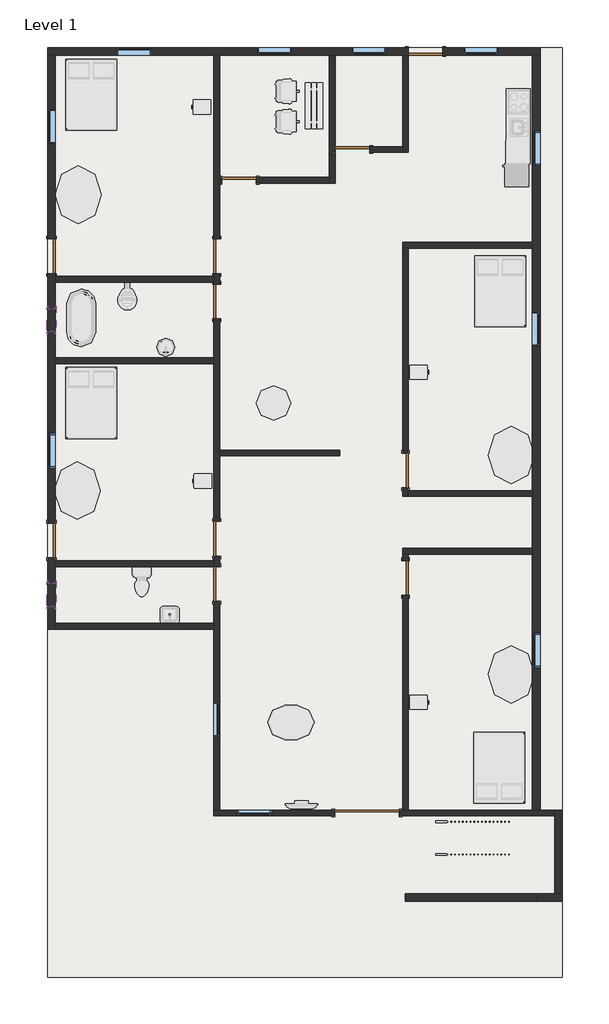
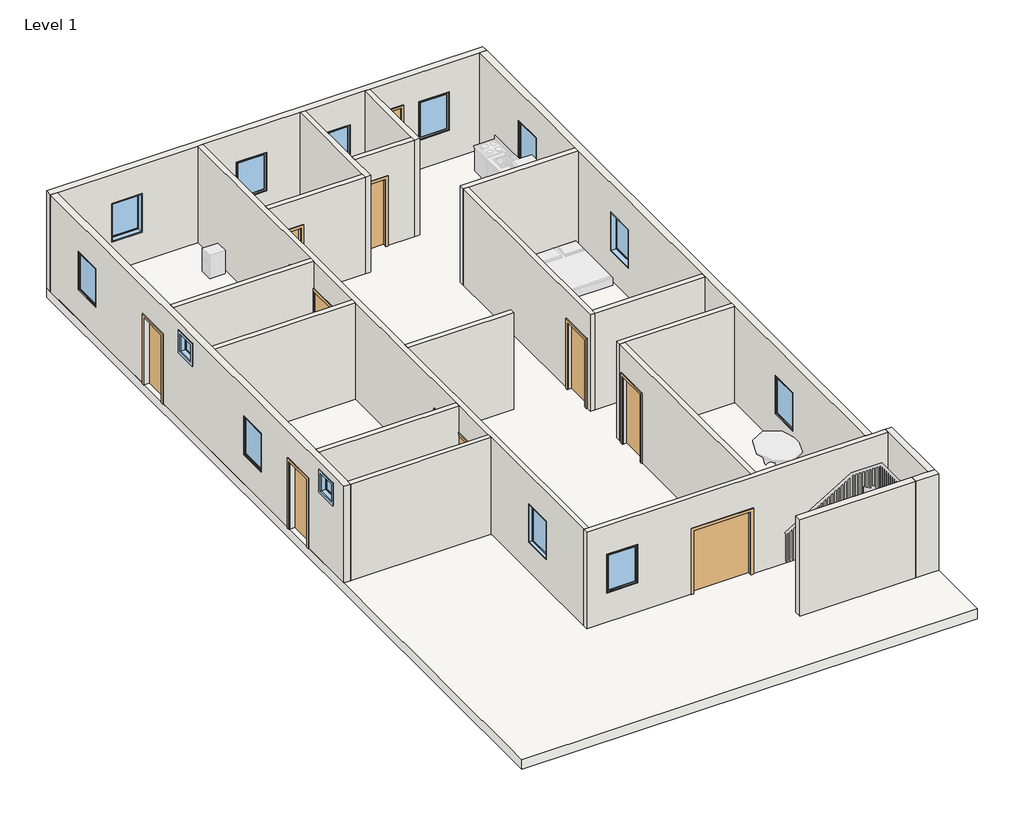
# One storey, part 1 of 2: 22 walls, 13 windows, 12 doors, 1 slab.
"""IFC4 building model written with IfcOpenShell, lengths in millimetres."""

from ifc_helpers import new_model, si_unit, frame, origin, origin_with_axes, place, context, project, spatial, polyline, outline, extrude, faceted_brep, transform, mapped, element, save
from components import m_door_double_flush_panel_double_acting_1700_x_2000mm_82a3dfda, door_54dd4da4, door_686f89d2, door_16372e1c, window_e2841890, window_d657a5cb, window_e41d21a6

model = new_model("IFC4")

# Units and contexts
model_context = context("Model", 3, world=origin())
ifc_project = project(units=[si_unit("LENGTHUNIT", "METRE", prefix="MILLI")], contexts=[model_context])

# Site, building, storey
site = spatial("IfcSite", under=ifc_project)
building = spatial("IfcBuilding", under=site)
storey = spatial("IfcBuildingStorey", under=building, Name="Level 1", Elevation=0.0)

# Doors
placement = place(None, origin())
m_door_double_flush_panel_double_acting_1700_x_2000mm_shape = m_door_double_flush_panel_double_acting_1700_x_2000mm_82a3dfda(model_context)
element("IfcDoor", 1, ObjectType="M_Door-Double-Flush_Panel-Double-Acting : 1700 x 2000mm", at=placement, inside=storey, context=model_context, shape_type="MappedRepresentation", body=[
    mapped(m_door_double_flush_panel_double_acting_1700_x_2000mm_shape, transform((-10492.7409023, -9232.8133562, 0.0), x_axis=(1.0, 0.0, 0.0), y_axis=(0.0, 1.0, 0.0), z_axis=(0.0, 0.0, 1.0))),
])
door_shape = door_54dd4da4(model_context)
element("IfcDoor", 2, ObjectType="Single-Flush : 36\" x 84\"", at=placement, inside=storey, context=model_context, shape_type="MappedRepresentation", body=[
    mapped(door_shape, transform((-18823.9409023, 5462.5226537, 0.0), x_axis=(0.0, -1.0, 0.0), y_axis=(1.0, 0.0, 0.0), z_axis=(0.0, 0.0, 1.0))),
])
element("IfcDoor", 3, ObjectType="Single-Flush : 36\" x 84\"", at=placement, inside=storey, context=model_context, shape_type="MappedRepresentation", body=[
    mapped(door_shape, transform((-8943.3409023, 10872.7226537, 0.0), x_axis=(-1.0, 0.0, 0.0), y_axis=(0.0, -1.0, 0.0), z_axis=(0.0, 0.0, 1.0))),
])
element("IfcDoor", 4, ObjectType="Single-Flush : 36\" x 84\"", at=placement, inside=storey, context=model_context, shape_type="MappedRepresentation", body=[
    mapped(door_shape, transform((-18823.9409023, -2044.6133562, 0.0), x_axis=(0.0, -1.0, 0.0), y_axis=(1.0, 0.0, 0.0), z_axis=(0.0, 0.0, 1.0))),
])
door_2_shape = door_686f89d2(model_context)
element("IfcDoor", 5, ObjectType="Single-Flush : 36\" x 84\"", at=placement, inside=storey, context=model_context, shape_type="MappedRepresentation", body=[
    mapped(door_2_shape, transform((-14455.1409023, 5462.5226537, 0.0), x_axis=(0.0, -1.0, 0.0), y_axis=(1.0, 0.0, 0.0), z_axis=(0.0, 0.0, 1.0))),
])
element("IfcDoor", 6, ObjectType="Single-Flush : 36\" x 84\"", at=placement, inside=storey, context=model_context, shape_type="MappedRepresentation", body=[
    mapped(door_2_shape, transform((-13870.9409023, 7469.1226537, 0.0), x_axis=(-1.0, 0.0, 0.0), y_axis=(0.0, -1.0, 0.0), z_axis=(0.0, 0.0, 1.0))),
])
element("IfcDoor", 7, ObjectType="Single-Flush : 36\" x 84\"", at=placement, inside=storey, context=model_context, shape_type="MappedRepresentation", body=[
    mapped(door_2_shape, transform((-10873.7409023, 8281.9226537, 0.0), x_axis=(-1.0, 0.0, 0.0), y_axis=(0.0, -1.0, 0.0), z_axis=(0.0, 0.0, 1.0))),
])
element("IfcDoor", 8, ObjectType="Single-Flush : 36\" x 84\"", at=placement, inside=storey, context=model_context, shape_type="MappedRepresentation", body=[
    mapped(door_2_shape, transform((-14455.1409023, -1993.8133562, 0.0), x_axis=(0.0, -1.0, 0.0), y_axis=(1.0, 0.0, 0.0), z_axis=(0.0, 0.0, 1.0))),
])
element("IfcDoor", 9, ObjectType="Single-Flush : 36\" x 84\"", at=placement, inside=storey, context=model_context, shape_type="MappedRepresentation", body=[
    mapped(door_2_shape, transform((-9476.7409023, -3035.2133562, 0.0), x_axis=(0.0, 1.0, 0.0), y_axis=(-1.0, 0.0, 0.0), z_axis=(0.0, 0.0, 1.0))),
])
door_3_shape = door_16372e1c(model_context)
element("IfcDoor", 10, ObjectType="Single-Flush : 36\" x 84\"", at=placement, inside=storey, context=model_context, shape_type="MappedRepresentation", body=[
    mapped(door_3_shape, transform((-9476.7409023, -190.4133562, 0.0), x_axis=(0.0, -1.0, 0.0), y_axis=(1.0, 0.0, 0.0), z_axis=(0.0, 0.0, 1.0))),
])
element("IfcDoor", 11, ObjectType="Single-Flush : 36\" x 84\"", at=placement, inside=storey, context=model_context, shape_type="MappedRepresentation", body=[
    mapped(door_3_shape, transform((-14455.1409023, 4268.7226537, 0.0), x_axis=(0.0, 1.0, 0.0), y_axis=(-1.0, 0.0, 0.0), z_axis=(0.0, 0.0, 1.0))),
])
element("IfcDoor", 12, ObjectType="Single-Flush : 36\" x 84\"", at=placement, inside=storey, context=model_context, shape_type="MappedRepresentation", body=[
    mapped(door_3_shape, transform((-14455.1409023, -3187.6133562, 0.0), x_axis=(0.0, 1.0, 0.0), y_axis=(-1.0, 0.0, 0.0), z_axis=(0.0, 0.0, 1.0))),
])

# Slab
element("IfcSlab", 13, ObjectType="Generic - 12\"", at=placement, inside=storey, context=model_context, shape_type="SweptSolid", body=[
    extrude(outline(polyline([(-5336.5409023, 10974.3226537), (-5336.5409023, -13576.2133562), (-18925.5409023, -13576.2133562), (-18925.5409023, 10974.3226537), (-5336.5409023, 10974.3226537)])), frame((0.0, 0.0, -304.8), z_axis=(0.0, 0.0, 1.0), x_axis=(1.0, 0.0, 0.0)), (0.0, 0.0, 1.0), 304.8),
])

# Walls
element("IfcWall", 14, ObjectType="Generic - 8\"", at=placement, inside=storey, context=model_context, shape_type="Brep", body=[
    faceted_brep([(-18925.5409023, 10771.1226537, 0.0), (-18722.3409023, 10771.1226537, 0.0), (-14531.3409023, 10771.1226537, 0.0), (-14378.9409023, 10771.1226537, 0.0), (-11483.3409023, 10771.1226537, 0.0), (-11330.9409023, 10771.1226537, 0.0), (-9552.9409023, 10771.1226537, 0.0), (-9400.5409023, 10771.1226537, 0.0), (-9400.5409023, 10771.1226537, 2133.6), (-8486.1409023, 10771.1226537, 2133.6), (-8486.1409023, 10771.1226537, 0.0), (-6123.9409023, 10771.1226537, 0.0), (-5920.7409023, 10771.1226537, 0.0), (-5920.7409023, 10771.1226537, 3048.0), (-6123.9409023, 10771.1226537, 3048.0), (-9400.5409023, 10771.1226537, 3048.0), (-9552.9409023, 10771.1226537, 3048.0), (-11330.9409023, 10771.1226537, 3048.0), (-11483.3409023, 10771.1226537, 3048.0), (-14378.9409023, 10771.1226537, 3048.0), (-14531.3409023, 10771.1226537, 3048.0), (-18722.3409023, 10771.1226537, 3048.0), (-18925.5409023, 10771.1226537, 3048.0), (-16182.3409023, 10771.1226537, 2133.6), (-16182.3409023, 10771.1226537, 914.4), (-17096.7409023, 10771.1226537, 914.4), (-17096.7409023, 10771.1226537, 2133.6), (-13388.3409023, 10771.1226537, 2133.6), (-12473.9409023, 10771.1226537, 2133.6), (-12473.9409023, 10771.1226537, 914.4), (-13388.3409023, 10771.1226537, 914.4), (-10899.1409023, 10771.1226537, 2133.6), (-9984.7409023, 10771.1226537, 2133.6), (-9984.7409023, 10771.1226537, 914.4), (-10899.1409023, 10771.1226537, 914.4), (-7940.0409023, 10771.1226537, 2133.6), (-7025.6409023, 10771.1226537, 2133.6), (-7025.6409023, 10771.1226537, 914.4), (-7940.0409023, 10771.1226537, 914.4), (-9400.5409023, 10974.3226537, 2133.6), (-9400.5409023, 10974.3226537, 0.0), (-18925.5409023, 10974.3226537, 0.0), (-18925.5409023, 10974.3226537, 3048.0), (-5920.7409023, 10974.3226537, 3048.0), (-5920.7409023, 10974.3226537, 0.0), (-8486.1409023, 10974.3226537, 0.0), (-8486.1409023, 10974.3226537, 2133.6), (-16182.3409023, 10974.3226537, 2133.6), (-17096.7409023, 10974.3226537, 2133.6), (-17096.7409023, 10974.3226537, 914.4), (-16182.3409023, 10974.3226537, 914.4), (-13388.3409023, 10974.3226537, 2133.6), (-13388.3409023, 10974.3226537, 914.4), (-12473.9409023, 10974.3226537, 914.4), (-12473.9409023, 10974.3226537, 2133.6), (-10899.1409023, 10974.3226537, 2133.6), (-10899.1409023, 10974.3226537, 914.4), (-9984.7409023, 10974.3226537, 914.4), (-9984.7409023, 10974.3226537, 2133.6), (-7940.0409023, 10974.3226537, 2133.6), (-7940.0409023, 10974.3226537, 914.4), (-7025.6409023, 10974.3226537, 914.4), (-7025.6409023, 10974.3226537, 2133.6)], [[[0, 1, 2, 3, 4, 5, 6, 7, 8, 9, 10, 11, 12, 13, 14, 15, 16, 17, 18, 19, 20, 21, 22], [23, 24, 25, 26], [27, 28, 29, 30], [31, 32, 33, 34], [35, 36, 37, 38]], [[39, 40, 41, 42, 43, 44, 45, 46], [47, 48, 49, 50], [51, 52, 53, 54], [55, 56, 57, 58], [59, 60, 61, 62]], [[45, 44, 12, 11, 10]], [[41, 40, 7, 6, 5, 4, 3, 2, 1, 0]], [[22, 21, 20, 19, 18, 17, 16, 15, 14, 13, 43, 42]], [[0, 22, 42, 41]], [[13, 12, 44, 43]], [[8, 7, 40, 39]], [[9, 8, 39, 46]], [[10, 9, 46, 45]], [[24, 23, 47, 50]], [[25, 24, 50, 49]], [[26, 25, 49, 48]], [[23, 26, 48, 47]], [[52, 51, 27, 30]], [[53, 52, 30, 29]], [[54, 53, 29, 28]], [[51, 54, 28, 27]], [[56, 55, 31, 34]], [[57, 56, 34, 33]], [[58, 57, 33, 32]], [[55, 58, 32, 31]], [[60, 59, 35, 38]], [[61, 60, 38, 37]], [[62, 61, 37, 36]], [[59, 62, 36, 35]]]),
])
element("IfcWall", 15, ObjectType="Generic - 8\"", at=placement, inside=storey, context=model_context, shape_type="Brep", body=[
    faceted_brep([(-18925.5409023, -2501.8133562, 2133.6), (-18925.5409023, -2501.8133562, 0.0), (-18925.5409023, -4381.4133562, 0.0), (-18925.5409023, -4381.4133562, 3048.0), (-18925.5409023, 10771.1226537, 3048.0), (-18925.5409023, 10771.1226537, 0.0), (-18925.5409023, 5919.7226537, 0.0), (-18925.5409023, 5919.7226537, 2133.6), (-18925.5409023, 5005.3226537, 2133.6), (-18925.5409023, 5005.3226537, 0.0), (-18925.5409023, -1587.4133562, 0.0), (-18925.5409023, -1587.4133562, 2133.6), (-18925.5409023, 9348.7226537, 2133.6), (-18925.5409023, 8434.3226537, 2133.6), (-18925.5409023, 8434.3226537, 914.4), (-18925.5409023, 9348.7226537, 914.4), (-18925.5409023, 787.4866438, 2133.6), (-18925.5409023, -126.9133562, 2133.6), (-18925.5409023, -126.9133562, 914.4), (-18925.5409023, 787.4866438, 914.4), (-18925.5409023, 3474.2546488, 2768.6), (-18925.5409023, 3474.2546488, 2159.0), (-18925.5409023, 4083.8546488, 2159.0), (-18925.5409023, 4083.8546488, 2768.6), (-18925.5409023, -3784.5133562, 2768.6), (-18925.5409023, -3784.5133562, 2159.0), (-18925.5409023, -3174.9133562, 2159.0), (-18925.5409023, -3174.9133562, 2768.6), (-18722.3409023, -4381.4133562, 0.0), (-18722.3409023, -4229.0133562, 0.0), (-18722.3409023, -2730.4133562, 0.0), (-18722.3409023, -2578.0133562, 0.0), (-18722.3409023, -2501.8133562, 0.0), (-18722.3409023, -2501.8133562, 2133.6), (-18722.3409023, -1587.4133562, 2133.6), (-18722.3409023, -1587.4133562, 0.0), (-18722.3409023, 2628.9866438, 0.0), (-18722.3409023, 2781.3866438, 0.0), (-18722.3409023, 4776.7226537, 0.0), (-18722.3409023, 4929.1226537, 0.0), (-18722.3409023, 5005.3226537, 0.0), (-18722.3409023, 5005.3226537, 2133.6), (-18722.3409023, 5919.7226537, 2133.6), (-18722.3409023, 5919.7226537, 0.0), (-18722.3409023, 10771.1226537, 0.0), (-18722.3409023, 10771.1226537, 3048.0), (-18722.3409023, 4929.1226537, 3048.0), (-18722.3409023, 4776.7226537, 3048.0), (-18722.3409023, 2781.3866438, 3048.0), (-18722.3409023, 2628.9866438, 3048.0), (-18722.3409023, -2578.0133562, 3048.0), (-18722.3409023, -2730.4133562, 3048.0), (-18722.3409023, -4229.0133562, 3048.0), (-18722.3409023, -4381.4133562, 3048.0), (-18722.3409023, 9348.7226537, 2133.6), (-18722.3409023, 9348.7226537, 914.4), (-18722.3409023, 8434.3226537, 914.4), (-18722.3409023, 8434.3226537, 2133.6), (-18722.3409023, 787.4866438, 2133.6), (-18722.3409023, 787.4866438, 914.4), (-18722.3409023, -126.9133562, 914.4), (-18722.3409023, -126.9133562, 2133.6), (-18722.3409023, 3474.2546488, 2768.6), (-18722.3409023, 4083.8546488, 2768.6), (-18722.3409023, 4083.8546488, 2159.0), (-18722.3409023, 3474.2546488, 2159.0), (-18722.3409023, -3784.5133562, 2768.6), (-18722.3409023, -3174.9133562, 2768.6), (-18722.3409023, -3174.9133562, 2159.0), (-18722.3409023, -3784.5133562, 2159.0)], [[[0, 1, 2, 3, 4, 5, 6, 7, 8, 9, 10, 11], [12, 13, 14, 15], [16, 17, 18, 19], [20, 21, 22, 23], [24, 25, 26, 27]], [[28, 29, 30, 31, 32, 33, 34, 35, 36, 37, 38, 39, 40, 41, 42, 43, 44, 45, 46, 47, 48, 49, 50, 51, 52, 53], [54, 55, 56, 57], [58, 59, 60, 61], [62, 63, 64, 65], [66, 67, 68, 69]], [[6, 5, 44, 43]], [[10, 9, 40, 39, 38, 37, 36, 35]], [[2, 1, 32, 31, 30, 29, 28]], [[4, 3, 53, 52, 51, 50, 49, 48, 47, 46, 45]], [[5, 4, 45, 44]], [[3, 2, 28, 53]], [[41, 40, 9, 8]], [[42, 41, 8, 7]], [[43, 42, 7, 6]], [[33, 32, 1, 0]], [[34, 33, 0, 11]], [[35, 34, 11, 10]], [[55, 54, 12, 15]], [[56, 55, 15, 14]], [[57, 56, 14, 13]], [[54, 57, 13, 12]], [[59, 58, 16, 19]], [[60, 59, 19, 18]], [[61, 60, 18, 17]], [[58, 61, 17, 16]], [[21, 20, 62, 65]], [[22, 21, 65, 64]], [[23, 22, 64, 63]], [[20, 23, 63, 62]], [[25, 24, 66, 69]], [[26, 25, 69, 68]], [[27, 26, 68, 67]], [[24, 27, 67, 66]]]),
])
element("IfcWall", 16, ObjectType="Generic - 8\"", at=placement, inside=storey, context=model_context, shape_type="Brep", body=[
    faceted_brep([(-5920.7409023, -9156.6133562, 0.0), (-5920.7409023, 10771.1226537, 0.0), (-5920.7409023, 10771.1226537, 3048.0), (-5920.7409023, -9156.6133562, 3048.0), (-5920.7409023, -4483.0133562, 2133.6), (-5920.7409023, -4483.0133562, 914.4), (-5920.7409023, -5397.4133562, 914.4), (-5920.7409023, -5397.4133562, 2133.6), (-5920.7409023, 8770.1546488, 2133.6), (-5920.7409023, 8770.1546488, 914.4), (-5920.7409023, 7855.7546488, 914.4), (-5920.7409023, 7855.7546488, 2133.6), (-5920.7409023, 3086.1866438, 2133.6), (-5920.7409023, 4000.5866438, 2133.6), (-5920.7409023, 4000.5866438, 914.4), (-5920.7409023, 3086.1866438, 914.4), (-6123.9409023, -9156.6133562, 0.0), (-6123.9409023, -9156.6133562, 3048.0), (-6123.9409023, -2400.2133562, 3048.0), (-6123.9409023, -2247.8133562, 3048.0), (-6123.9409023, -876.2133562, 3048.0), (-6123.9409023, -723.8133562, 3048.0), (-6123.9409023, 5676.9866438, 3048.0), (-6123.9409023, 5829.3866438, 3048.0), (-6123.9409023, 10771.1226537, 3048.0), (-6123.9409023, 10771.1226537, 0.0), (-6123.9409023, 5829.3866438, 0.0), (-6123.9409023, 5676.9866438, 0.0), (-6123.9409023, -723.8133562, 0.0), (-6123.9409023, -876.2133562, 0.0), (-6123.9409023, -2247.8133562, 0.0), (-6123.9409023, -2400.2133562, 0.0), (-6123.9409023, -4483.0133562, 2133.6), (-6123.9409023, -5397.4133562, 2133.6), (-6123.9409023, -5397.4133562, 914.4), (-6123.9409023, -4483.0133562, 914.4), (-6123.9409023, 8770.1546488, 2133.6), (-6123.9409023, 7855.7546488, 2133.6), (-6123.9409023, 7855.7546488, 914.4), (-6123.9409023, 8770.1546488, 914.4), (-6123.9409023, 3086.1866438, 2133.6), (-6123.9409023, 3086.1866438, 914.4), (-6123.9409023, 4000.5866438, 914.4), (-6123.9409023, 4000.5866438, 2133.6)], [[[0, 1, 2, 3], [4, 5, 6, 7], [8, 9, 10, 11], [12, 13, 14, 15]], [[16, 17, 18, 19, 20, 21, 22, 23, 24, 25, 26, 27, 28, 29, 30, 31], [32, 33, 34, 35], [36, 37, 38, 39], [40, 41, 42, 43]], [[1, 0, 16, 31, 30, 29, 28, 27, 26, 25]], [[3, 2, 24, 23, 22, 21, 20, 19, 18, 17]], [[0, 3, 17, 16]], [[5, 4, 32, 35]], [[6, 5, 35, 34]], [[7, 6, 34, 33]], [[4, 7, 33, 32]], [[8, 11, 37, 36]], [[11, 10, 38, 37]], [[10, 9, 39, 38]], [[9, 8, 36, 39]], [[40, 43, 13, 12]], [[43, 42, 14, 13]], [[42, 41, 15, 14]], [[41, 40, 12, 15]], [[2, 1, 25, 24]]]),
])
element("IfcWall", 17, ObjectType="Generic - 8\"", at=placement, inside=storey, context=model_context, shape_type="SweptSolid", body=[
    extrude(outline(polyline([(-6022.3409023, -11569.6133562), (-9476.7409023, -11569.6133562), (-9476.7409023, -11366.4133562), (-6022.3409023, -11366.4133562), (-6022.3409023, -11569.6133562)])), origin_with_axes(), (0.0, 0.0, 1.0), 3048.0),
])
element("IfcWall", 18, ObjectType="Generic - 8\"", at=placement, inside=storey, context=model_context, shape_type="Brep", body=[
    faceted_brep([(-5336.5409023, -11366.4133562, 0.0), (-5336.5409023, -9156.6133562, 0.0), (-5336.5409023, -9156.6133562, 3048.0), (-5336.5409023, -11366.4133562, 3048.0), (-5539.7409023, -11366.4133562, 0.0), (-5539.7409023, -11366.4133562, 3048.0), (-5539.7409023, -9309.0133562, 3048.0), (-5539.7409023, -9156.6133562, 3048.0), (-5539.7409023, -9156.6133562, 0.0), (-5539.7409023, -9309.0133562, 0.0)], [[[0, 1, 2, 3]], [[4, 5, 6, 7, 8, 9]], [[1, 0, 4, 9, 8]], [[3, 2, 7, 6, 5]], [[0, 3, 5, 4]], [[2, 1, 8, 7]]]),
])
element("IfcWall", 19, ObjectType="Generic - 8\"", at=placement, inside=storey, context=model_context, shape_type="Brep", body=[
    faceted_brep([(-6022.3409023, -11569.6133562, 0.0), (-5336.5409023, -11569.6133562, 0.0), (-5336.5409023, -11569.6133562, 3048.0), (-6022.3409023, -11569.6133562, 3048.0), (-6022.3409023, -11366.4133562, 0.0), (-6022.3409023, -11366.4133562, 3048.0), (-5539.7409023, -11366.4133562, 3048.0), (-5336.5409023, -11366.4133562, 3048.0), (-5336.5409023, -11366.4133562, 0.0), (-5539.7409023, -11366.4133562, 0.0)], [[[0, 1, 2, 3]], [[4, 5, 6, 7, 8, 9]], [[1, 0, 4, 9, 8]], [[3, 2, 7, 6, 5]], [[0, 3, 5, 4]], [[2, 1, 8, 7]]]),
])
element("IfcWall", 20, ObjectType="inner Generic - 6\"", at=placement, inside=storey, context=model_context, shape_type="Brep", body=[
    faceted_brep([(-14531.3409023, -2451.0133562, 0.0), (-14531.3409023, -2578.0133562, 0.0), (-14531.3409023, -2730.4133562, 0.0), (-14531.3409023, -2730.4133562, 2133.6), (-14531.3409023, -3644.8133562, 2133.6), (-14531.3409023, -3644.8133562, 0.0), (-14531.3409023, -4229.0133562, 0.0), (-14531.3409023, -4381.4133562, 0.0), (-14531.3409023, -9156.6133562, 0.0), (-14531.3409023, -9156.6133562, 3048.0), (-14531.3409023, -4381.4133562, 3048.0), (-14531.3409023, -4229.0133562, 3048.0), (-14531.3409023, -2730.4133562, 3048.0), (-14531.3409023, -2578.0133562, 3048.0), (-14531.3409023, 2628.9866438, 3048.0), (-14531.3409023, 2781.3866438, 3048.0), (-14531.3409023, 4776.7226537, 3048.0), (-14531.3409023, 4929.1226537, 3048.0), (-14531.3409023, 10771.1226537, 3048.0), (-14531.3409023, 10771.1226537, 0.0), (-14531.3409023, 5919.7226537, 0.0), (-14531.3409023, 5919.7226537, 2133.6), (-14531.3409023, 5005.3226537, 2133.6), (-14531.3409023, 5005.3226537, 0.0), (-14531.3409023, 4929.1226537, 0.0), (-14531.3409023, 4776.7226537, 0.0), (-14531.3409023, 4725.9226537, 0.0), (-14531.3409023, 4725.9226537, 2133.6), (-14531.3409023, 3811.5226537, 2133.6), (-14531.3409023, 3811.5226537, 0.0), (-14531.3409023, 2781.3866438, 0.0), (-14531.3409023, 2628.9866438, 0.0), (-14531.3409023, -1536.6133562, 0.0), (-14531.3409023, -1536.6133562, 2133.6), (-14531.3409023, -2451.0133562, 2133.6), (-14531.3409023, -7226.2133562, 2133.6), (-14531.3409023, -7226.2133562, 914.4), (-14531.3409023, -6311.8133562, 914.4), (-14531.3409023, -6311.8133562, 2133.6), (-14378.9409023, -2730.4133562, 2133.6), (-14378.9409023, -2730.4133562, 0.0), (-14378.9409023, -2451.0133562, 0.0), (-14378.9409023, -2451.0133562, 2133.6), (-14378.9409023, -1536.6133562, 2133.6), (-14378.9409023, -1536.6133562, 0.0), (-14378.9409023, 190.5866438, 0.0), (-14378.9409023, 342.9866438, 0.0), (-14378.9409023, 3811.5226537, 0.0), (-14378.9409023, 3811.5226537, 2133.6), (-14378.9409023, 4725.9226537, 2133.6), (-14378.9409023, 4725.9226537, 0.0), (-14378.9409023, 5005.3226537, 0.0), (-14378.9409023, 5005.3226537, 2133.6), (-14378.9409023, 5919.7226537, 2133.6), (-14378.9409023, 5919.7226537, 0.0), (-14378.9409023, 7392.9226537, 0.0), (-14378.9409023, 7545.3226537, 0.0), (-14378.9409023, 10771.1226537, 0.0), (-14378.9409023, 10771.1226537, 3048.0), (-14378.9409023, 7545.3226537, 3048.0), (-14378.9409023, 7392.9226537, 3048.0), (-14378.9409023, 342.9866438, 3048.0), (-14378.9409023, 190.5866438, 3048.0), (-14378.9409023, -9156.6133562, 3048.0), (-14378.9409023, -9156.6133562, 0.0), (-14378.9409023, -3644.8133562, 0.0), (-14378.9409023, -3644.8133562, 2133.6), (-14378.9409023, -7226.2133562, 2133.6), (-14378.9409023, -6311.8133562, 2133.6), (-14378.9409023, -6311.8133562, 914.4), (-14378.9409023, -7226.2133562, 914.4)], [[[0, 1, 2, 3, 4, 5, 6, 7, 8, 9, 10, 11, 12, 13, 14, 15, 16, 17, 18, 19, 20, 21, 22, 23, 24, 25, 26, 27, 28, 29, 30, 31, 32, 33, 34], [35, 36, 37, 38]], [[39, 40, 41, 42, 43, 44, 45, 46, 47, 48, 49, 50, 51, 52, 53, 54, 55, 56, 57, 58, 59, 60, 61, 62, 63, 64, 65, 66], [67, 68, 69, 70]], [[20, 19, 57, 56, 55, 54]], [[51, 50, 26, 25, 24, 23]], [[65, 64, 8, 7, 6, 5]], [[41, 40, 2, 1, 0]], [[47, 46, 45, 44, 32, 31, 30, 29]], [[18, 17, 16, 15, 14, 13, 12, 11, 10, 9, 63, 62, 61, 60, 59, 58]], [[19, 18, 58, 57]], [[52, 51, 23, 22]], [[53, 52, 22, 21]], [[54, 53, 21, 20]], [[44, 43, 33, 32]], [[43, 42, 34, 33]], [[42, 41, 0, 34]], [[9, 8, 64, 63]], [[27, 26, 50, 49]], [[28, 27, 49, 48]], [[29, 28, 48, 47]], [[3, 2, 40, 39]], [[4, 3, 39, 66]], [[5, 4, 66, 65]], [[36, 35, 67, 70]], [[37, 36, 70, 69]], [[38, 37, 69, 68]], [[35, 38, 68, 67]]]),
])
element("IfcWall", 21, ObjectType="inner Generic - 6\"", at=placement, inside=storey, context=model_context, shape_type="SweptSolid", body=[
    extrude(outline(polyline([(-18722.3409023, 4929.1226537), (-14531.3409023, 4929.1226537), (-14531.3409023, 4776.7226537), (-18722.3409023, 4776.7226537), (-18722.3409023, 4929.1226537)])), origin_with_axes(), (0.0, 0.0, 1.0), 3048.0),
])
element("IfcWall", 22, ObjectType="inner Generic - 6\"", at=placement, inside=storey, context=model_context, shape_type="Brep", body=[
    faceted_brep([(-11483.3409023, 10771.1226537, 0.0), (-11483.3409023, 7545.3226537, 0.0), (-11483.3409023, 7392.9226537, 0.0), (-11483.3409023, 7392.9226537, 3048.0), (-11483.3409023, 7545.3226537, 3048.0), (-11483.3409023, 10771.1226537, 3048.0), (-11330.9409023, 10771.1226537, 0.0), (-11330.9409023, 10771.1226537, 3048.0), (-11330.9409023, 8358.1226537, 3048.0), (-11330.9409023, 8205.7226537, 3048.0), (-11330.9409023, 7392.9226537, 3048.0), (-11330.9409023, 7392.9226537, 0.0)], [[[0, 1, 2, 3, 4, 5]], [[6, 7, 8, 9, 10, 11]], [[2, 1, 0, 6, 11]], [[5, 4, 3, 10, 9, 8, 7]], [[0, 5, 7, 6]], [[3, 2, 11, 10]]]),
])
element("IfcWall", 23, ObjectType="inner Generic - 6\"", at=placement, inside=storey, context=model_context, shape_type="SweptSolid", body=[
    extrude(outline(polyline([(0.0, -14378.9409023), (0.0, -14328.1409023), (2133.6, -14328.1409023), (2133.6, -13413.7409023), (0.0, -13413.7409023), (0.0, -11483.3409023), (3048.0, -11483.3409023), (3048.0, -14378.9409023), (0.0, -14378.9409023)])), frame((0.0, 7392.9226537, 0.0), z_axis=(0.0, 1.0, 0.0), x_axis=(0.0, 0.0, 1.0)), (0.0, 0.0, 1.0), 152.4),
])
element("IfcWall", 24, ObjectType="inner Generic - 6\"", at=placement, inside=storey, context=model_context, shape_type="Brep", body=[
    faceted_brep([(-9552.9409023, 10771.1226537, 0.0), (-9552.9409023, 8358.1226537, 0.0), (-9552.9409023, 8205.7226537, 0.0), (-9552.9409023, 8205.7226537, 3048.0), (-9552.9409023, 8358.1226537, 3048.0), (-9552.9409023, 10771.1226537, 3048.0), (-9400.5409023, 10771.1226537, 0.0), (-9400.5409023, 10771.1226537, 3048.0), (-9400.5409023, 8205.7226537, 3048.0), (-9400.5409023, 8205.7226537, 0.0)], [[[0, 1, 2, 3, 4, 5]], [[6, 7, 8, 9]], [[2, 1, 0, 6, 9]], [[5, 4, 3, 8, 7]], [[0, 5, 7, 6]], [[3, 2, 9, 8]]]),
])
element("IfcWall", 25, ObjectType="inner Generic - 6\"", at=placement, inside=storey, context=model_context, shape_type="SweptSolid", body=[
    extrude(outline(polyline([(3048.0, -9552.9409023), (3048.0, -11330.9409023), (2133.6, -11330.9409023), (2133.6, -10416.5409023), (0.0, -10416.5409023), (0.0, -9552.9409023), (3048.0, -9552.9409023)])), frame((0.0, 8205.7226537, 0.0), z_axis=(0.0, 1.0, 0.0), x_axis=(0.0, 0.0, 1.0)), (0.0, 0.0, 1.0), 152.4),
])
element("IfcWall", 26, ObjectType="inner Generic - 6\"", at=placement, inside=storey, context=model_context, shape_type="Brep", body=[
    faceted_brep([(-9552.9409023, 5676.9866438, 0.0), (-9400.5409023, 5676.9866438, 0.0), (-6123.9409023, 5676.9866438, 0.0), (-6123.9409023, 5676.9866438, 3048.0), (-9400.5409023, 5676.9866438, 3048.0), (-9552.9409023, 5676.9866438, 3048.0), (-9552.9409023, 5829.3866438, 0.0), (-9552.9409023, 5829.3866438, 3048.0), (-6123.9409023, 5829.3866438, 3048.0), (-6123.9409023, 5829.3866438, 0.0)], [[[0, 1, 2, 3, 4, 5]], [[6, 7, 8, 9]], [[2, 1, 0, 6, 9]], [[5, 4, 3, 8, 7]], [[3, 2, 9, 8]], [[0, 5, 7, 6]]]),
])
element("IfcWall", 27, ObjectType="inner Generic - 6\"", at=placement, inside=storey, context=model_context, shape_type="Brep", body=[
    faceted_brep([(-9552.9409023, -647.6133562, 2133.6), (-9552.9409023, -647.6133562, 0.0), (-9552.9409023, -876.2133562, 0.0), (-9552.9409023, -876.2133562, 3048.0), (-9552.9409023, 5676.9866438, 3048.0), (-9552.9409023, 5676.9866438, 0.0), (-9552.9409023, 266.7866438, 0.0), (-9552.9409023, 266.7866438, 2133.6), (-9400.5409023, -876.2133562, 0.0), (-9400.5409023, -723.8133562, 0.0), (-9400.5409023, -647.6133562, 0.0), (-9400.5409023, -647.6133562, 2133.6), (-9400.5409023, 266.7866438, 2133.6), (-9400.5409023, 266.7866438, 0.0), (-9400.5409023, 5676.9866438, 0.0), (-9400.5409023, 5676.9866438, 3048.0), (-9400.5409023, -723.8133562, 3048.0), (-9400.5409023, -876.2133562, 3048.0)], [[[0, 1, 2, 3, 4, 5, 6, 7]], [[8, 9, 10, 11, 12, 13, 14, 15, 16, 17]], [[6, 5, 14, 13]], [[2, 1, 10, 9, 8]], [[4, 3, 17, 16, 15]], [[5, 4, 15, 14]], [[3, 2, 8, 17]], [[11, 10, 1, 0]], [[12, 11, 0, 7]], [[13, 12, 7, 6]]]),
])
element("IfcWall", 28, ObjectType="inner Generic - 6\"", at=placement, inside=storey, context=model_context, shape_type="SweptSolid", body=[
    extrude(outline(polyline([(-6123.9409023, -876.2133562), (-9400.5409023, -876.2133562), (-9400.5409023, -723.8133562), (-6123.9409023, -723.8133562), (-6123.9409023, -876.2133562)])), origin_with_axes(), (0.0, 0.0, 1.0), 3048.0),
])
element("IfcWall", 29, ObjectType="inner Generic - 6\"", at=placement, inside=storey, context=model_context, shape_type="Brep", body=[
    faceted_brep([(-9552.9409023, -2400.2133562, 0.0), (-9400.5409023, -2400.2133562, 0.0), (-6123.9409023, -2400.2133562, 0.0), (-6123.9409023, -2400.2133562, 3048.0), (-9400.5409023, -2400.2133562, 3048.0), (-9552.9409023, -2400.2133562, 3048.0), (-9552.9409023, -2247.8133562, 0.0), (-9552.9409023, -2247.8133562, 3048.0), (-6123.9409023, -2247.8133562, 3048.0), (-6123.9409023, -2247.8133562, 0.0)], [[[0, 1, 2, 3, 4, 5]], [[6, 7, 8, 9]], [[2, 1, 0, 6, 9]], [[5, 4, 3, 8, 7]], [[3, 2, 9, 8]], [[0, 5, 7, 6]]]),
])
element("IfcWall", 30, ObjectType="inner Generic - 6\"", at=placement, inside=storey, context=model_context, shape_type="SweptSolid", body=[
    extrude(outline(polyline([(-9156.6133562, 3048.0), (-2400.2133562, 3048.0), (-2400.2133562, 0.0), (-2578.0133562, 0.0), (-2578.0133562, 2133.6), (-3492.4133562, 2133.6), (-3492.4133562, 0.0), (-9156.6133562, 0.0), (-9156.6133562, 3048.0)])), frame((-9552.9409023, 0.0, 0.0), z_axis=(1.0, 0.0, 0.0), x_axis=(0.0, 1.0, 0.0)), (0.0, 0.0, 1.0), 152.4),
])
element("IfcWall", 31, ObjectType="inner Generic - 6\"", at=placement, inside=storey, context=model_context, shape_type="Brep", body=[
    faceted_brep([(-5539.7409023, -9309.0133562, 3048.0), (-14531.3409023, -9309.0133562, 3048.0), (-14531.3409023, -9309.0133562, 0.0), (-11342.7409023, -9309.0133562, 0.0), (-11342.7409023, -9309.0133562, 2000.0), (-9642.7409023, -9309.0133562, 2000.0), (-9642.7409023, -9309.0133562, 0.0), (-5539.7409023, -9309.0133562, 0.0), (-13921.7409023, -9309.0133562, 2133.6), (-13007.3409023, -9309.0133562, 2133.6), (-13007.3409023, -9309.0133562, 914.4), (-13921.7409023, -9309.0133562, 914.4), (-14531.3409023, -9156.6133562, 3048.0), (-14378.9409023, -9156.6133562, 3048.0), (-9552.9409023, -9156.6133562, 3048.0), (-9400.5409023, -9156.6133562, 3048.0), (-6123.9409023, -9156.6133562, 3048.0), (-5920.7409023, -9156.6133562, 3048.0), (-5539.7409023, -9156.6133562, 3048.0), (-5539.7409023, -9156.6133562, 0.0), (-5920.7409023, -9156.6133562, 0.0), (-6123.9409023, -9156.6133562, 0.0), (-9400.5409023, -9156.6133562, 0.0), (-9552.9409023, -9156.6133562, 0.0), (-9642.7409023, -9156.6133562, 0.0), (-9642.7409023, -9156.6133562, 2000.0), (-11342.7409023, -9156.6133562, 2000.0), (-11342.7409023, -9156.6133562, 0.0), (-14378.9409023, -9156.6133562, 0.0), (-14531.3409023, -9156.6133562, 0.0), (-13921.7409023, -9156.6133562, 2133.6), (-13921.7409023, -9156.6133562, 914.4), (-13007.3409023, -9156.6133562, 914.4), (-13007.3409023, -9156.6133562, 2133.6)], [[[0, 1, 2, 3, 4, 5, 6, 7], [8, 9, 10, 11]], [[12, 13, 14, 15, 16, 17, 18, 19, 20, 21, 22, 23, 24, 25, 26, 27, 28, 29], [30, 31, 32, 33]], [[2, 29, 28, 27, 3]], [[19, 7, 6, 24, 23, 22, 21, 20]], [[1, 0, 18, 17, 16, 15, 14, 13, 12]], [[2, 1, 12, 29]], [[5, 25, 24, 6]], [[25, 5, 4, 26]], [[26, 4, 3, 27]], [[31, 30, 8, 11]], [[32, 31, 11, 10]], [[33, 32, 10, 9]], [[30, 33, 9, 8]], [[0, 7, 19, 18]]]),
])
element("IfcWall", 32, ObjectType="inner Generic - 6\"", at=placement, inside=storey, context=model_context, shape_type="SweptSolid", body=[
    extrude(outline(polyline([(-18722.3409023, -4229.0133562), (-14531.3409023, -4229.0133562), (-14531.3409023, -4381.4133562), (-18722.3409023, -4381.4133562), (-18722.3409023, -4229.0133562)])), origin_with_axes(), (0.0, 0.0, 1.0), 3048.0),
])
element("IfcWall", 33, ObjectType="inner Generic - 6\"", at=placement, inside=storey, context=model_context, shape_type="SweptSolid", body=[
    extrude(outline(polyline([(-18722.3409023, -2578.0133562), (-14531.3409023, -2578.0133562), (-14531.3409023, -2730.4133562), (-18722.3409023, -2730.4133562), (-18722.3409023, -2578.0133562)])), origin_with_axes(), (0.0, 0.0, 1.0), 3048.0),
])
element("IfcWall", 34, ObjectType="inner Generic - 6\"", at=placement, inside=storey, context=model_context, shape_type="SweptSolid", body=[
    extrude(outline(polyline([(-18722.3409023, 2781.3866438), (-14531.3409023, 2781.3866438), (-14531.3409023, 2628.9866438), (-18722.3409023, 2628.9866438), (-18722.3409023, 2781.3866438)])), origin_with_axes(), (0.0, 0.0, 1.0), 3048.0),
])
element("IfcWall", 35, ObjectType="inner Generic - 6\"", at=placement, inside=storey, context=model_context, shape_type="SweptSolid", body=[
    extrude(outline(polyline([(-11216.6409023, 190.5866438), (-14378.9409023, 190.5866438), (-14378.9409023, 342.9866438), (-11216.6409023, 342.9866438), (-11216.6409023, 190.5866438)])), origin_with_axes(), (0.0, 0.0, 1.0), 3048.0),
])

# Windows
window_shape = window_e2841890(model_context)
element("IfcWindow", 36, ObjectType="Fixed : 36\" x 48\"", at=placement, inside=storey, context=model_context, shape_type="MappedRepresentation", body=[
    mapped(window_shape, transform((-16601.4409023, 10872.7226537, 0.0), x_axis=(1.0, 0.0, 0.0), y_axis=(0.0, 1.0, 0.0), z_axis=(0.0, 0.0, 1.0))),
])
element("IfcWindow", 37, ObjectType="Fixed : 36\" x 48\"", at=placement, inside=storey, context=model_context, shape_type="MappedRepresentation", body=[
    mapped(window_shape, transform((-18823.9409023, 8929.6226537, 0.0), x_axis=(0.0, 1.0, 0.0), y_axis=(-1.0, 0.0, 0.0), z_axis=(0.0, 0.0, 1.0))),
])
element("IfcWindow", 38, ObjectType="Fixed : 36\" x 48\"", at=placement, inside=storey, context=model_context, shape_type="MappedRepresentation", body=[
    mapped(window_shape, transform((-12969.2409023, 10872.7226537, 0.0), x_axis=(-1.0, 0.0, 0.0), y_axis=(0.0, -1.0, 0.0), z_axis=(0.0, 0.0, 1.0))),
])
element("IfcWindow", 39, ObjectType="Fixed : 36\" x 48\"", at=placement, inside=storey, context=model_context, shape_type="MappedRepresentation", body=[
    mapped(window_shape, transform((-10480.0409023, 10872.7226537, 0.0), x_axis=(-1.0, 0.0, 0.0), y_axis=(0.0, -1.0, 0.0), z_axis=(0.0, 0.0, 1.0))),
])
element("IfcWindow", 40, ObjectType="Fixed : 36\" x 48\"", at=placement, inside=storey, context=model_context, shape_type="MappedRepresentation", body=[
    mapped(window_shape, transform((-7520.9409023, 10872.7226537, 0.0), x_axis=(-1.0, 0.0, 0.0), y_axis=(0.0, -1.0, 0.0), z_axis=(0.0, 0.0, 1.0))),
])
element("IfcWindow", 41, ObjectType="Fixed : 36\" x 48\"", at=placement, inside=storey, context=model_context, shape_type="MappedRepresentation", body=[
    mapped(window_shape, transform((-6022.3409023, 8351.0546488, 0.0), x_axis=(0.0, 1.0, 0.0), y_axis=(-1.0, 0.0, 0.0), z_axis=(0.0, 0.0, 1.0))),
])
element("IfcWindow", 42, ObjectType="Fixed : 36\" x 48\"", at=placement, inside=storey, context=model_context, shape_type="MappedRepresentation", body=[
    mapped(window_shape, transform((-6022.3409023, 3505.2866438, 0.0), x_axis=(0.0, -1.0, 0.0), y_axis=(1.0, 0.0, 0.0), z_axis=(0.0, 0.0, 1.0))),
])
element("IfcWindow", 43, ObjectType="Fixed : 36\" x 48\"", at=placement, inside=storey, context=model_context, shape_type="MappedRepresentation", body=[
    mapped(window_shape, transform((-6022.3409023, -4902.1133562, 0.0), x_axis=(0.0, 1.0, 0.0), y_axis=(-1.0, 0.0, 0.0), z_axis=(0.0, 0.0, 1.0))),
])
element("IfcWindow", 44, ObjectType="Fixed : 36\" x 48\"", at=placement, inside=storey, context=model_context, shape_type="MappedRepresentation", body=[
    mapped(window_shape, transform((-18823.9409023, 368.3866438, 0.0), x_axis=(0.0, 1.0, 0.0), y_axis=(-1.0, 0.0, 0.0), z_axis=(0.0, 0.0, 1.0))),
])
window_2_shape = window_d657a5cb(model_context)
element("IfcWindow", 45, ObjectType="Fixed : 36\" x 48\"", at=placement, inside=storey, context=model_context, shape_type="MappedRepresentation", body=[
    mapped(window_2_shape, transform((-13502.6409023, -9232.8133562, 0.0), x_axis=(-1.0, 0.0, 0.0), y_axis=(0.0, -1.0, 0.0), z_axis=(0.0, 0.0, 1.0))),
])
element("IfcWindow", 46, ObjectType="Fixed : 36\" x 48\"", at=placement, inside=storey, context=model_context, shape_type="MappedRepresentation", body=[
    mapped(window_2_shape, transform((-14455.1409023, -6807.1133562, 0.0), x_axis=(0.0, -1.0, 0.0), y_axis=(1.0, 0.0, 0.0), z_axis=(0.0, 0.0, 1.0))),
])
window_3_shape = window_e41d21a6(model_context)
element("IfcWindow", 47, ObjectType="Transom with Trim : 24\" x 24\"", at=placement, inside=storey, context=model_context, shape_type="MappedRepresentation", body=[
    mapped(window_3_shape, transform((-18823.9409023, 3740.9546488, 0.0), x_axis=(0.0, -1.0, 0.0), y_axis=(1.0, 0.0, 0.0), z_axis=(0.0, 0.0, 1.0))),
])
element("IfcWindow", 48, ObjectType="Transom with Trim : 24\" x 24\"", at=placement, inside=storey, context=model_context, shape_type="MappedRepresentation", body=[
    mapped(window_3_shape, transform((-18823.9409023, -3517.8133562, 0.0), x_axis=(0.0, -1.0, 0.0), y_axis=(1.0, 0.0, 0.0), z_axis=(0.0, 0.0, 1.0))),
])

save(model, "model.ifc")

# Revit data of these elements
# Type "M_Door-Double-Flush_Panel-Double-Acting : 1700 x 2000mm"
#   Type Mark = "8"
#   Construction Type Id = "DOOR"
#   Assembly Code = "C1020"
#   Analytic Construction = "Wooden"
#   W = 2' - 9.46457"
#   Thickness = 0' - 1.9685"
#   Thermal Resistance (R) = 2.5876 (h·ft²·°F)/BTU
#   Swing Angle [instance default] = 90.00°
#   Heat Transfer Coefficient (U) = 0.3865 BTU/(h·ft²·°F)
#   Height = 6' - 6.74016"
#   Trim Projection Ext. = 0' - 0.98425"
#   Trim Projection Int. = 0' - 0.98425"
#   Trim Width Ext. = 0' - 3.14961"
#   Trim Width Int. = 0' - 3.14961"
#   Width = 5' - 6.92913"
#   Define Thermal Properties by = 1
#   Panel Material = Wood - Birch - Solid Stained Light Low Gloss
#   Trim Material = Paint - Sienna
#   Visual Light Transmittance = 0
#   Solar Heat Gain Coefficient = 0
#   Function = (empty or 0)
#   Wall Closure = (empty or 0)
# Type "Single-Flush : 36\" x 84\""
#   Type Mark = "1"
#   Construction Type Id = "MDOOR"
#   Assembly Code = "C1020"
#   Analytic Construction = "Metal"
#   Thickness = 0' - 2"
#   Heat Transfer Coefficient (U) = 0.651978 BTU/(h·ft²·°F)
#   Height = 7' - 0"
#   Trim Projection Ext = 0' - 1"
#   Trim Projection Int = 0' - 1"
#   Trim Width = 0' - 3"
#   Width = 3' - 0"
#   Define Thermal Properties by = 1
#   Door Material = Door - Panel
#   Frame Material = Door - Frame
#   Visual Light Transmittance = 0
#   Solar Heat Gain Coefficient = 0
#   Function = (empty or 0)
#   Wall Closure = (empty or 0)
# Type "Generic - 12\""
#   Assembly Code = "B1010"
#   Function = 0
#   Layers, outside or top first: 1' - 0" no material (function 1)
# Type "Generic - 8\""
#   Assembly Code = "B2010"
#   Layers, outside or top first: 0' - 8" no material (function 1)
# Type "inner Generic - 6\""
#   Assembly Code = "B2010"
#   Layers, outside or top first: 0' - 6" no material (function 1)
# Type "Fixed : 36\" x 48\""
#   Type Mark = "1"
#   Construction Type Id = "GSP4R"
#   Assembly Code = "B2020100"
#   Analytic Construction = "1/8 in Pilkington single glazing"
#   Visual Light Transmittance = 0.9
#   Solar Heat Gain Coefficient = 0.78
#   Heat Transfer Coefficient (U) = 0.6496 BTU/(h·ft²·°F)
#   Height = 4' - 0"
#   Default Sill Height = 3' - 0"
#   Width = 3' - 0"
#   Window Inset = 0' - 0 3/4"
#   Define Thermal Properties by = 1
#   Glass Pane Material = Glass
#   Sash Material = Sash
#   Wall Closure = (empty or 0)
# Type "Transom with Trim : 24\" x 24\""
#   Type Mark = "10"
#   Construction Type Id = "GSP4R"
#   Assembly Code = "B2020100"
#   Analytic Construction = "1/8 in Pilkington single glazing"
#   Visual Light Transmittance = 0.9
#   Solar Heat Gain Coefficient = 0.78
#   Heat Transfer Coefficient (U) = 0.6496 BTU/(h·ft²·°F)
#   Height = 2' - 0"
#   Default Sill Height = 7' - 1"
#   Trim Projection - Ext. = 0' - 0 1/2"
#   Trim Projection - Int. = 0' - 0 3/4"
#   Trim Width - Exterior = 0' - 3 1/2"
#   Trim Width - Interior = 0' - 3 1/2"
#   Width = 2' - 0"
#   Window Inset = 0' - 0 3/4"
#   Define Thermal Properties by = 1
#   Glass Pane Material = Glass
#   Sash Material = Sash
#   Trim Exterior Material = Trim
#   Trim Interior Material = Trim
#   Wall Closure = (empty or 0)
# Element 1 (IfcDoor, "M_Door-Double-Flush_Panel-Double-Acting : 1700 x 2000mm")
#   Swing Angle = 90.00°
#   Phase Created = New Construction
#   Materials on its faces: "Paint - Sienna", "Wood - Birch - Solid Stained Light Low Gloss"
# Elements 2, 3, 4, 5, 6, 7, 8, 9, 10, 11, 12 (IfcDoor, "Single-Flush : 36\" x 84\"")
#   Phase Created = New Construction
#   Materials on its faces: "Door - Frame", "Door - Panel"
# Element 13 (IfcSlab, "Generic - 12\"")
#   Height Offset From Level = 0' - 0"
#   Phase Created = New Construction
#   Materials on its faces: "Default Floor"
# Elements 14, 15, 16, 17, 18, 19 (IfcWall, "Generic - 8\"")
#   Top Offset = 0' - 0"
#   Base Offset = 0' - 0"
#   Unconnected Height = 10' - 0"
#   wall height = 10' - 0"
#   Phase Created = New Construction
#   Base Constraint = Level 1
#   Materials on its faces: "Default Wall"
# Elements 20, 21, 22, 23, 24, 25, 26, 27, 28, 29, 30, 31, 32, 33, 34, 35 (IfcWall, "inner Generic - 6\"")
#   Top Offset = 0' - 0"
#   Base Offset = 0' - 0"
#   Unconnected Height = 10' - 0"
#   wall height = 10' - 0"
#   Phase Created = New Construction
#   Base Constraint = Level 1
#   Materials on its faces: "Default Wall"
# Element 36 (IfcWindow, "Fixed : 36\" x 48\"")
#   Mark = "1"
#   Phase Created = New Construction
#   Materials on its faces: "Sash", "Glass"
# Element 37 (IfcWindow, "Fixed : 36\" x 48\"")
#   Mark = "2"
#   Phase Created = New Construction
#   Materials on its faces: "Sash", "Glass"
# Element 38 (IfcWindow, "Fixed : 36\" x 48\"")
#   Mark = "3"
#   Phase Created = New Construction
#   Materials on its faces: "Sash", "Glass"
# Element 39 (IfcWindow, "Fixed : 36\" x 48\"")
#   Mark = "4"
#   Phase Created = New Construction
#   Materials on its faces: "Sash", "Glass"
# Element 40 (IfcWindow, "Fixed : 36\" x 48\"")
#   Mark = "5"
#   Phase Created = New Construction
#   Materials on its faces: "Sash", "Glass"
# Element 41 (IfcWindow, "Fixed : 36\" x 48\"")
#   Mark = "6"
#   Phase Created = New Construction
#   Materials on its faces: "Sash", "Glass"
# Element 42 (IfcWindow, "Fixed : 36\" x 48\"")
#   Mark = "7"
#   Phase Created = New Construction
#   Materials on its faces: "Sash", "Glass"
# Element 43 (IfcWindow, "Fixed : 36\" x 48\"")
#   Mark = "8"
#   Phase Created = New Construction
#   Materials on its faces: "Sash", "Glass"
# Element 44 (IfcWindow, "Fixed : 36\" x 48\"")
#   Mark = "11"
#   Phase Created = New Construction
#   Materials on its faces: "Sash", "Glass"
# Element 45 (IfcWindow, "Fixed : 36\" x 48\"")
#   Mark = "9"
#   Phase Created = New Construction
#   Materials on its faces: "Sash", "Glass"
# Element 46 (IfcWindow, "Fixed : 36\" x 48\"")
#   Mark = "10"
#   Phase Created = New Construction
#   Materials on its faces: "Sash", "Glass"
# Element 47 (IfcWindow, "Transom with Trim : 24\" x 24\"")
#   Mark = "12"
#   Phase Created = New Construction
#   Materials on its faces: "Sash", "Trim", "Glass"
# Element 48 (IfcWindow, "Transom with Trim : 24\" x 24\"")
#   Mark = "13"
#   Phase Created = New Construction
#   Materials on its faces: "Sash", "Trim", "Glass"
# Materials
#   "Wood - Birch - Solid Stained Light Low Gloss": class "Wood", colour RGB 210 159 95, transparency 0, Cost = 0
#   "Paint - Sienna": colour RGB 118 70 51, transparency 0, Cost = 0
#   "Door - Panel": class "Wood", colour RGB 210 159 95, transparency 0
#   "Door - Frame": colour RGB 118 70 51, transparency 0
#   "Glass": class "Glass", colour RGB 0 128 192, transparency 0.75, Description = "Soda Lime Glass", Cost = 0
#   "Sash": class "Wood", colour RGB 224 178 126, transparency 0
#   "Trim": class "Wood", colour RGB 224 178 126, transparency 0
#   "Default Floor": colour RGB 128 128 128, transparency 0
#   "Default Wall": colour RGB 128 128 128, transparency 0
# Room at (-16127.007, 7923.101) mm, phase "New Construction", upper level "Level 1", upper offset 10' - 0", lower offset 0' - 0"
#   Number = "1"
#   Name = "BED ROOM 1"
# Room at (-12877.167, 9185.256) mm, phase "New Construction", upper level "Level 1", upper offset 10' - 0", lower offset 0' - 0"
#   Number = "2"
#   Name = "STUDY ROOM"
# Room at (-10429.235, 9185.256) mm, phase "New Construction", upper level "Level 1", upper offset 10' - 0", lower offset 0' - 0"
#   Number = "3"
# Room at (-7939.098, 7923.101) mm, phase "New Construction", upper level "Level 1", upper offset 10' - 0", lower offset 0' - 0"
#   Number = "4"
#   Name = "KITCHEN"
# Room at (-16127.007, 3744.735) mm, phase "New Construction", upper level "Level 1", upper offset 10' - 0", lower offset 0' - 0"
#   Number = "5"
# Room at (-16127.007, 0) mm, phase "New Construction", upper level "Level 1", upper offset 10' - 0", lower offset 0' - 0"
#   Number = "6"
#   Name = "BED ROOM 2"
# Room at (-16127.007, -2881.563) mm, phase "New Construction", upper level "Level 1", upper offset 10' - 0", lower offset 0' - 0"
#   Number = "7"
# Room at (-12258.035, -5076.26) mm, phase "New Construction", upper level "Level 1", upper offset 10' - 0", lower offset 0' - 0"
#   Number = "8"
#   Name = "LIVING ROOM"
# Room at (-7939.098, -5751.552) mm, phase "New Construction", upper level "Level 1", upper offset 10' - 0", lower offset 0' - 0"
#   Number = "9"
#   Name = "BED ROOM 4"
# Room at (-7939.098, 1929.889) mm, phase "New Construction", upper level "Level 1", upper offset 10' - 0", lower offset 0' - 0"
#   Number = "10"
#   Name = "BED ROOM 3"
# Room at (-12258.035, 3744.735) mm, phase "New Construction", upper level "Level 1", upper offset 10' - 0", lower offset 0' - 0"
#   Number = "11"
# Room at (-7352.594, -1798.625) mm, phase "New Construction", upper level "Level 1", upper offset 10' - 0", lower offset 0' - 0"
#   Number = "12"
